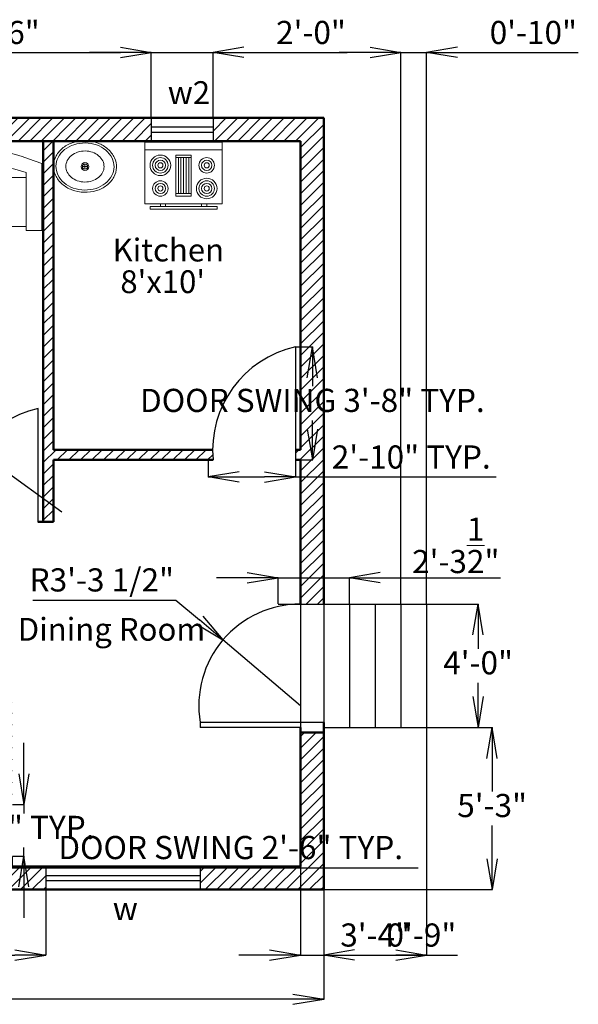
# Model space of a CAD drawing. Units: inches. Extents: x 1856 to 3350, y 1624 to 2224.
# Tile 3 of 7: x 2159 to 2376, y 1782 to 2165. Entities that reach past the tile are written whole.
import ezdxf

# ---------------------------------------------------------------- set-up
doc = ezdxf.new("R2010")
doc.units = ezdxf.units.IN
for name, color, linetype, lineweight in [('A-ANNO-DIMS', 2, 'Continuous', 18), ('A-ANNO-TEXT', 7, 'Continuous', 18), ('A-AREA-IDEN', 7, 'Continuous', 25), ('A-DOOR', 3, 'Continuous', 25), ('A-EQPM', 3, 'Continuous', 18), ('A-FLOR-FIXT', 3, 'Continuous', 18), ('A-FLOR-STRS', 7, 'Continuous', 25), ('A-FURN', 3, 'Continuous', 18), ('A-WALL', 7, 'Continuous', 50), ('A-WALL-PATT', 8, 'Continuous', 13), ('window', 4, 'Continuous', 25)]:
    doc.layers.add(name, color=color, linetype=linetype, lineweight=lineweight)
doc.styles.get("Standard").update_dxf_attribs({"font": 'arial.ttf'})
doc.dimstyles.new('ISO-25', dxfattribs={"dimtxt": 9, "dimasz": 12, "dimexe": 0.125, "dimexo": 0.125, "dimgap": 2, "dimtad": 1, "dimtih": 1, "dimtoh": 1, "dimdec": 1, "dimzin": 11, "dimlunit": 4, "dimtxsty": 'Standard', "dimblk": 'OPEN', "dimcen": -0.125, "dimadec": 0, "dimazin": 0, "dimtfac": 1, "dimtdec": 1, "dimtmove": 0, "dimatfit": 3, "dimfxl": 1, "dimarcsym": 0})

# ---------------------------------------------------------------- blocks, each defined once
blk = doc.blocks.new('_Open')
at = {"color": 0, "linetype": 'ByBlock', "lineweight": -2}
for p, q in [((-1, 0.167), (0, 0)), ((-1, -0.167), (0, 0)), ((0, 0), (-1, 0))]:
    blk.add_line(p, q, dxfattribs=at)
blk = doc.blocks.new('*D2')
at = {"layer": 'A-ANNO-DIMS', "color": 0, "lineweight": -2, "transparency": 16777216}
for p, q in [((2317.24, 1937.99), (2337.23, 1937.99)), ((2337.11, 1925.99), (2337.11, 1920.59)), ((2337.11, 1901.99), (2337.11, 1907.4)), ((2317.24, 1889.99), (2337.23, 1889.99))]:
    blk.add_line(p, q, dxfattribs=at)
at = {"layer": 'Defpoints', "color": 0, "transparency": 16777216}
for p in [(2317.11, 1937.99), (2317.11, 1889.99), (2337.11, 1889.99)]:
    blk.add_point(p, dxfattribs=at)
at = {"layer": 'A-ANNO-DIMS', "color": 0, "lineweight": -2, "transparency": 16777216, "xscale": 12, "yscale": 12, "zscale": 12}
for p, rotation in [((2337.11, 1937.99), 90), ((2337.11, 1889.99), 270)]:
    blk.add_blockref('_Open', p, dxfattribs=dict(at, rotation=rotation))
at = {"layer": 'A-ANNO-DIMS', "color": 0, "transparency": 16777216, "insert": (2337.11, 1913.99), "char_height": 9, "attachment_point": 5}
blk.add_mtext('4\'-0"', dxfattribs=at)
blk = doc.blocks.new('*D3')
at = {"layer": 'A-ANNO-DIMS', "color": 0, "lineweight": -2, "transparency": 16777216}
for p, q in [((2247.41, 1948.19), (2235.41, 1948.19)), ((2259.41, 1938.12), (2259.41, 1948.31)), ((2259.41, 1948.19), (2287.11, 1948.19)), ((2287.11, 1938.12), (2287.11, 1948.31)), ((2299.11, 1948.19), (2345.75, 1948.19))]:
    blk.add_line(p, q, dxfattribs=at)
at = {"layer": 'Defpoints', "color": 0, "transparency": 16777216}
for p in [(2287.11, 1948.19), (2259.41, 1937.99), (2287.11, 1937.99)]:
    blk.add_point(p, dxfattribs=at)
at = {"layer": 'A-ANNO-DIMS', "color": 0, "lineweight": -2, "transparency": 16777216, "xscale": 12, "yscale": 12, "zscale": 12}
blk.add_blockref('_Open', (2259.41, 1948.19), dxfattribs=at)
at = {"layer": 'A-ANNO-DIMS', "color": 0, "lineweight": -2, "transparency": 16777216, "xscale": 12, "yscale": 12, "zscale": 12, "rotation": 180}
blk.add_blockref('_Open', (2287.11, 1948.19), dxfattribs=at)
at = {"layer": 'A-ANNO-DIMS', "color": 0, "transparency": 16777216, "insert": (2328.43, 1960.81), "char_height": 9, "attachment_point": 5}
blk.add_mtext('2\'-3{\\H1x;\\S1/2;}"', dxfattribs=at)
blk = doc.blocks.new('*D7')
at = {"layer": 'A-ANNO-DIMS', "color": 0, "lineweight": -2, "transparency": 16777216}
for p, q in [((1923.11, 1826.87), (1923.11, 1784.25)), ((2277.11, 1826.87), (2277.11, 1784.25)), ((2265.11, 1784.37), (1935.11, 1784.37))]:
    blk.add_line(p, q, dxfattribs=at)
at = {"layer": 'Defpoints', "color": 0, "transparency": 16777216}
for p in [(1923.11, 1826.99), (2277.11, 1826.99), (1923.11, 1784.37)]:
    blk.add_point(p, dxfattribs=at)
at = {"layer": 'A-ANNO-DIMS', "color": 0, "lineweight": -2, "transparency": 16777216, "xscale": 12, "yscale": 12, "zscale": 12, "rotation": 180}
blk.add_blockref('_Open', (1923.11, 1784.37), dxfattribs=at)
at = {"layer": 'A-ANNO-DIMS', "color": 0, "lineweight": -2, "transparency": 16777216, "xscale": 12, "yscale": 12, "zscale": 12}
blk.add_blockref('_Open', (2277.11, 1784.37), dxfattribs=at)
at = {"layer": 'A-ANNO-DIMS', "color": 0, "transparency": 16777216, "insert": (2100.11, 1790.97), "char_height": 9, "attachment_point": 5}
blk.add_mtext("30'", dxfattribs=at)
blk = doc.blocks.new('Range-Oven - 30 in top')
for p, q in [((0, -3), (30, -3)), ((12, -6), (18, -6)), ((13, -20), (13, -6)), ((14, -6), (14, -20)), ((15, -20), (15, -6)), ((16, -6), (16, -20)), ((17, -20), (17, -6)), ((18, -20), (12, -20)), ((6, -24), (6, -25)), ((8, -25), (8, -24)), ((22, -25), (22, -24)), ((24, -24), (24, -25))]:
    blk.add_line(p, q)
for points in [[(0, -24), (0, 0), (30, 0), (30, -24)], [(12, -21), (12, -5), (18, -5), (18, -21)], [(2, -26), (2, -25), (28, -25), (28, -26)]]:
    blk.add_lwpolyline(points, close=True)
for centre, radius in [((6, -9), 4), ((6, -9), 3), ((6, -9), 2), ((24, -9), 3), ((24, -9), 2), ((6, -9), 1), ((24, -9), 1), ((6, -18), 3), ((24, -18), 4), ((24, -18), 3), ((6, -18), 2), ((6, -18), 1), ((24, -18), 2), ((24, -18), 1)]:
    blk.add_circle(centre, radius)
blk = doc.blocks.new('Sink - Oval top')
for p, q in [((-1, 0), (1, 0)), ((0, 1), (0, -1))]:
    blk.add_line(p, q)
for points in [[(-12.23, 0.39, 0.117634), (-11.46, -3.36, 0.104469), (-8.88, -6.8, 0.090016), (-5.08, -9.07, 0.08192), (-0.32, -10.02, 0.08192), (4.49, -9.38, 0.090016), (8.42, -7.36, 0.104469), (11.22, -4.09, 0.117634), (12.23, -0.39, 0.117634), (11.46, 3.36, 0.104469), (8.88, 6.8, 0.090016), (5.08, 9.07, 0.08192), (0.32, 10.02, 0.08192), (-4.49, 9.38, 0.090016), (-8.42, 7.36, 0.104469), (-11.22, 4.09, 0.117634)], [(-11.29, 0.16, 0.118622), (-10.52, -3.25, 0.104678), (-8.07, -6.36, 0.089562), (-4.54, -8.37, 0.081185), (-0.13, -9.15, 0.081185), (4.3, -8.49, 0.089562), (7.89, -6.58, 0.104678), (10.42, -3.55, 0.118622), (11.29, -0.16, 0.118622), (10.52, 3.25, 0.104678), (8.07, 6.36, 0.089562), (4.54, 8.37, 0.081185), (0.13, 9.15, 0.081185), (-4.3, 8.49, 0.089562), (-7.89, 6.58, 0.104678), (-10.42, 3.55, 0.118622)], [(-7.42, 0.08, 0.118283), (-6.91, -2.17, 0.104607), (-5.29, -4.21, 0.089718), (-2.97, -5.53, 0.081436), (-0.07, -6.04, 0.081436), (2.84, -5.59, 0.089718), (5.2, -4.33, 0.104607), (6.86, -2.32, 0.118283), (7.42, -0.08, 0.118283), (6.91, 2.17, 0.104607), (5.29, 4.21, 0.089718), (2.97, 5.53, 0.081436), (0.07, 6.04, 0.081436), (-2.84, 5.59, 0.089718), (-5.2, 4.33, 0.104607), (-6.86, 2.32, 0.118283)]]:
    blk.add_lwpolyline(points, format="xyb", close=True)
for radius in [1.5, 1]:
    blk.add_circle((0, 0), radius)
blk = doc.blocks.new('Sofa - Roundback 7 ft.')
for p, q in [((-12.00002, -32.4421), (-12.00003, -6.5971)), ((11.99997, -32.4421), (11.99998, -6.5971)), ((-36.000027, -34), (-36.000027, -11.4696)), ((35.99998, -34), (35.99998, -11.4696)), ((-35.999844, -13.3819), (35.9998, -13.3819)), ((-36.000027, -32.4421), (35.99998, -32.4421))]:
    blk.add_line(p, q)
for points in [[(-36.000027, -34), (-42.000027, -34), (-42.000027, -8)], [(41.99998, -8), (41.99998, -34), (35.99998, -34)]]:
    blk.add_lwpolyline(points)
for centre, radius, start, end in [((0, -114.25), 114.25, 68.43141, 111.5686), ((-0.00001, -127.1968), 121.1968, 72.72033, 107.2797)]:
    blk.add_arc(centre, radius, start, end)
blk = doc.blocks.new('WIN-60')
for p, q in [((0, 9), (60, 9)), ((0, 9), (0, 0)), ((60, 9), (60, 0)), ((0, 5.5), (60, 5.5)), ((0, 3.5), (60, 3.5)), ((0, 0), (60, 0))]:
    blk.add_line(p, q)
blk = doc.blocks.new('DOOR-SWING-44')
blk.add_line((32.16, 44), (32.16, 0))
blk.add_arc((41.37, 3.67), 41.37, 102.8606, 185.0846)
blk = doc.blocks.new('*D58')
at = {"layer": 'A-ANNO-DIMS', "color": 0, "lineweight": -2, "transparency": 16777216}
for p, q in [((2266.24, 2037.99), (2272.84, 2037.99)), ((2272.71, 2025.99), (2272.71, 2022.65)), ((2272.71, 2005.99), (2272.71, 2009.33)), ((2266.24, 1993.99), (2272.84, 1993.99))]:
    blk.add_line(p, q, dxfattribs=at)
at = {"layer": 'Defpoints', "color": 0, "transparency": 16777216}
for p in [(2266.11, 2037.99), (2272.71, 2037.99), (2266.11, 1993.99)]:
    blk.add_point(p, dxfattribs=at)
at = {"layer": 'A-ANNO-DIMS', "color": 0, "lineweight": -2, "transparency": 16777216, "xscale": 12, "yscale": 12, "zscale": 12}
for p, rotation in [((2272.71, 2037.99), 90), ((2272.71, 1993.99), 270)]:
    blk.add_blockref('_Open', p, dxfattribs=dict(at, rotation=rotation))
at = {"layer": 'A-ANNO-DIMS', "color": 0, "transparency": 16777216, "insert": (2272.71, 2015.99), "char_height": 9, "attachment_point": 5}
blk.add_mtext('DOOR SWING 3\'-8" TYP.', dxfattribs=at)
blk = doc.blocks.new('*D59')
at = {"layer": 'A-ANNO-DIMS', "color": 0, "lineweight": -2, "transparency": 16777216}
for p, q in [((2232.28, 1993.87), (2232.28, 1987.27)), ((2266.11, 1993.87), (2266.11, 1987.27)), ((2244.28, 1987.39), (2254.11, 1987.39)), ((2266.11, 1987.39), (2344.12, 1987.39))]:
    blk.add_line(p, q, dxfattribs=at)
at = {"layer": 'Defpoints', "color": 0, "transparency": 16777216}
for p in [(2232.28, 1993.99), (2266.11, 1993.99), (2266.11, 1987.39)]:
    blk.add_point(p, dxfattribs=at)
at = {"layer": 'A-ANNO-DIMS', "color": 0, "lineweight": -2, "transparency": 16777216, "xscale": 12, "yscale": 12, "zscale": 12, "rotation": 180}
blk.add_blockref('_Open', (2232.28, 1987.39), dxfattribs=at)
at = {"layer": 'A-ANNO-DIMS', "color": 0, "lineweight": -2, "transparency": 16777216, "xscale": 12, "yscale": 12, "zscale": 12}
blk.add_blockref('_Open', (2266.11, 1987.39), dxfattribs=at)
at = {"layer": 'A-ANNO-DIMS', "color": 0, "transparency": 16777216, "insert": (2311.12, 1993.99), "char_height": 9, "attachment_point": 5}
blk.add_mtext('2\'-10" TYP.', dxfattribs=at)
blk = doc.blocks.new('*D60')
at = {"layer": 'A-ANNO-DIMS', "color": 0, "lineweight": -2, "transparency": 16777216}
for p, q in [((2126.11, 1839.87), (2126.11, 1835.37)), ((2156.11, 1839.87), (2156.11, 1835.37)), ((2138.11, 1835.49), (2144.11, 1835.49)), ((2156.11, 1835.49), (2313.84, 1835.49))]:
    blk.add_line(p, q, dxfattribs=at)
at = {"layer": 'Defpoints', "color": 0, "transparency": 16777216}
for p in [(2126.11, 1839.99), (2156.11, 1839.99), (2156.11, 1835.49)]:
    blk.add_point(p, dxfattribs=at)
at = {"layer": 'A-ANNO-DIMS', "color": 0, "lineweight": -2, "transparency": 16777216, "xscale": 12, "yscale": 12, "zscale": 12, "rotation": 180}
blk.add_blockref('_Open', (2126.11, 1835.49), dxfattribs=at)
at = {"layer": 'A-ANNO-DIMS', "color": 0, "lineweight": -2, "transparency": 16777216, "xscale": 12, "yscale": 12, "zscale": 12}
blk.add_blockref('_Open', (2156.11, 1835.49), dxfattribs=at)
at = {"layer": 'A-ANNO-DIMS', "color": 0, "transparency": 16777216, "insert": (2240.97, 1842.15), "char_height": 9, "attachment_point": 5}
blk.add_mtext('DOOR SWING 2\'-6" TYP.', dxfattribs=at)
blk = doc.blocks.new('*D61')
at = {"layer": 'A-ANNO-DIMS', "color": 0, "lineweight": -2, "transparency": 16777216}
for p, q in [((2160.61, 1871.99), (2160.61, 1883.99)), ((2156.24, 1859.99), (2160.74, 1859.99)), ((2160.61, 1859.99), (2160.61, 1856.59)), ((2160.61, 1839.99), (2160.61, 1843.4)), ((2156.24, 1839.99), (2160.74, 1839.99)), ((2160.61, 1827.99), (2160.61, 1815.99))]:
    blk.add_line(p, q, dxfattribs=at)
at = {"layer": 'Defpoints', "color": 0, "transparency": 16777216}
for p in [(2156.11, 1859.99), (2160.61, 1859.99), (2156.11, 1839.99)]:
    blk.add_point(p, dxfattribs=at)
at = {"layer": 'A-ANNO-DIMS', "color": 0, "lineweight": -2, "transparency": 16777216, "xscale": 12, "yscale": 12, "zscale": 12}
for p, rotation in [((2160.61, 1859.99), 270), ((2160.61, 1839.99), 90)]:
    blk.add_blockref('_Open', p, dxfattribs=dict(at, rotation=rotation))
at = {"layer": 'A-ANNO-DIMS', "color": 0, "transparency": 16777216, "insert": (2160.61, 1849.99), "char_height": 9, "attachment_point": 5}
blk.add_mtext('1\'-8" TYP.', dxfattribs=at)
blk = doc.blocks.new('*D62')
at = {"layer": 'A-ANNO-DIMS', "color": 0, "lineweight": -2, "transparency": 16777216}
for p, q in [((2277.11, 1889.87), (2277.11, 1801.42)), ((2317.11, 1889.87), (2317.11, 1801.42)), ((2289.11, 1801.54), (2305.11, 1801.54))]:
    blk.add_line(p, q, dxfattribs=at)
at = {"layer": 'Defpoints', "color": 0, "transparency": 16777216}
for p in [(2277.11, 1889.99), (2317.11, 1889.99), (2317.11, 1801.54)]:
    blk.add_point(p, dxfattribs=at)
at = {"layer": 'A-ANNO-DIMS', "color": 0, "lineweight": -2, "transparency": 16777216, "xscale": 12, "yscale": 12, "zscale": 12, "rotation": 180}
blk.add_blockref('_Open', (2277.11, 1801.54), dxfattribs=at)
at = {"layer": 'A-ANNO-DIMS', "color": 0, "lineweight": -2, "transparency": 16777216, "xscale": 12, "yscale": 12, "zscale": 12}
blk.add_blockref('_Open', (2317.11, 1801.54), dxfattribs=at)
at = {"layer": 'A-ANNO-DIMS', "color": 0, "transparency": 16777216, "insert": (2297.11, 1808.14), "char_height": 9, "attachment_point": 5}
blk.add_mtext('3\'-4"', dxfattribs=at)
blk = doc.blocks.new('*D63')
at = {"layer": 'A-ANNO-DIMS', "color": 0, "lineweight": -2, "transparency": 16777216}
for p, q in [((2295.11, 2152.44), (2283.11, 2152.44)), ((2307.11, 1938.12), (2307.11, 2152.57)), ((2307.11, 2152.44), (2317.11, 2152.44)), ((2317.11, 1938.12), (2317.11, 2152.57)), ((2329.11, 2152.44), (2376.03, 2152.44))]:
    blk.add_line(p, q, dxfattribs=at)
at = {"layer": 'Defpoints', "color": 0, "transparency": 16777216}
for p in [(2317.11, 2152.44), (2307.11, 1937.99), (2317.11, 1937.99)]:
    blk.add_point(p, dxfattribs=at)
at = {"layer": 'A-ANNO-DIMS', "color": 0, "lineweight": -2, "transparency": 16777216, "xscale": 12, "yscale": 12, "zscale": 12}
blk.add_blockref('_Open', (2307.11, 2152.44), dxfattribs=at)
at = {"layer": 'A-ANNO-DIMS', "color": 0, "lineweight": -2, "transparency": 16777216, "xscale": 12, "yscale": 12, "zscale": 12, "rotation": 180}
blk.add_blockref('_Open', (2317.11, 2152.44), dxfattribs=at)
at = {"layer": 'A-ANNO-DIMS', "color": 0, "transparency": 16777216, "insert": (2358.57, 2159.04), "char_height": 9, "attachment_point": 5}
blk.add_mtext('0\'-10"', dxfattribs=at)
blk = doc.blocks.new('*D64')
at = {"layer": 'A-ANNO-DIMS', "color": 0, "lineweight": -2, "transparency": 16777216}
for p, q in [((2268.11, 1937.87), (2268.11, 1801.42)), ((2277.11, 1937.87), (2277.11, 1801.42)), ((2256.11, 1801.54), (2244.11, 1801.54)), ((2268.11, 1801.54), (2277.11, 1801.54)), ((2289.11, 1801.54), (2329.04, 1801.54))]:
    blk.add_line(p, q, dxfattribs=at)
at = {"layer": 'Defpoints', "color": 0, "transparency": 16777216}
for p in [(2268.11, 1937.99), (2277.11, 1937.99), (2277.11, 1801.54)]:
    blk.add_point(p, dxfattribs=at)
at = {"layer": 'A-ANNO-DIMS', "color": 0, "lineweight": -2, "transparency": 16777216, "xscale": 12, "yscale": 12, "zscale": 12}
blk.add_blockref('_Open', (2268.11, 1801.54), dxfattribs=at)
at = {"layer": 'A-ANNO-DIMS', "color": 0, "lineweight": -2, "transparency": 16777216, "xscale": 12, "yscale": 12, "zscale": 12, "rotation": 180}
blk.add_blockref('_Open', (2277.11, 1801.54), dxfattribs=at)
at = {"layer": 'A-ANNO-DIMS', "color": 0, "transparency": 16777216, "insert": (2315.08, 1808.14), "char_height": 9, "attachment_point": 5}
blk.add_mtext('0\'-9"', dxfattribs=at)
blk = doc.blocks.new('*D66')
at = {"layer": 'A-ANNO-DIMS', "color": 0, "lineweight": -2, "transparency": 16777216}
for p, q in [((2096.3, 2127.12), (2096.3, 2152.57)), ((2108.3, 2152.44), (2198.14, 2152.44)), ((2210.14, 2127.12), (2210.14, 2152.57))]:
    blk.add_line(p, q, dxfattribs=at)
at = {"layer": 'Defpoints', "color": 0, "transparency": 16777216}
for p in [(2210.14, 2152.44), (2096.3, 2126.99), (2210.14, 2126.99)]:
    blk.add_point(p, dxfattribs=at)
at = {"layer": 'A-ANNO-DIMS', "color": 0, "lineweight": -2, "transparency": 16777216, "xscale": 12, "yscale": 12, "zscale": 12, "rotation": 180}
blk.add_blockref('_Open', (2096.3, 2152.44), dxfattribs=at)
at = {"layer": 'A-ANNO-DIMS', "color": 0, "lineweight": -2, "transparency": 16777216, "xscale": 12, "yscale": 12, "zscale": 12}
blk.add_blockref('_Open', (2210.14, 2152.44), dxfattribs=at)
at = {"layer": 'A-ANNO-DIMS', "color": 0, "transparency": 16777216, "insert": (2153.22, 2159.04), "char_height": 9, "attachment_point": 5}
blk.add_mtext('9\'-6"', dxfattribs=at)
blk = doc.blocks.new('*D67')
at = {"layer": 'A-ANNO-DIMS', "color": 0, "lineweight": -2, "transparency": 16777216}
for p, q in [((2198.14, 2152.44), (2186.14, 2152.44)), ((2210.14, 2127.12), (2210.14, 2152.57)), ((2210.14, 2152.44), (2234.14, 2152.44)), ((2234.14, 2127.12), (2234.14, 2152.57)), ((2246.14, 2152.44), (2286.22, 2152.44))]:
    blk.add_line(p, q, dxfattribs=at)
at = {"layer": 'Defpoints', "color": 0, "transparency": 16777216}
for p in [(2234.14, 2152.44), (2210.14, 2126.99), (2234.14, 2126.99)]:
    blk.add_point(p, dxfattribs=at)
at = {"layer": 'A-ANNO-DIMS', "color": 0, "lineweight": -2, "transparency": 16777216, "xscale": 12, "yscale": 12, "zscale": 12}
blk.add_blockref('_Open', (2210.14, 2152.44), dxfattribs=at)
at = {"layer": 'A-ANNO-DIMS', "color": 0, "lineweight": -2, "transparency": 16777216, "xscale": 12, "yscale": 12, "zscale": 12, "rotation": 180}
blk.add_blockref('_Open', (2234.14, 2152.44), dxfattribs=at)
at = {"layer": 'A-ANNO-DIMS', "color": 0, "transparency": 16777216, "insert": (2272.18, 2159.04), "char_height": 9, "attachment_point": 5}
blk.add_mtext('2\'-0"', dxfattribs=at)
blk = doc.blocks.new('*D70')
at = {"layer": 'A-ANNO-DIMS', "color": 0, "lineweight": -2, "transparency": 16777216}
for p, q in [((2104.11, 1826.87), (2104.11, 1801.42)), ((2169.11, 1826.87), (2169.11, 1801.42)), ((2116.11, 1801.54), (2157.11, 1801.54))]:
    blk.add_line(p, q, dxfattribs=at)
at = {"layer": 'Defpoints', "color": 0, "transparency": 16777216}
for p in [(2104.11, 1826.99), (2169.11, 1826.99), (2169.11, 1801.54)]:
    blk.add_point(p, dxfattribs=at)
at = {"layer": 'A-ANNO-DIMS', "color": 0, "lineweight": -2, "transparency": 16777216, "xscale": 12, "yscale": 12, "zscale": 12, "rotation": 180}
blk.add_blockref('_Open', (2104.11, 1801.54), dxfattribs=at)
at = {"layer": 'A-ANNO-DIMS', "color": 0, "lineweight": -2, "transparency": 16777216, "xscale": 12, "yscale": 12, "zscale": 12}
blk.add_blockref('_Open', (2169.11, 1801.54), dxfattribs=at)
at = {"layer": 'A-ANNO-DIMS', "color": 0, "transparency": 16777216, "insert": (2136.61, 1808.12), "char_height": 9, "attachment_point": 5}
blk.add_mtext('5\'-5"', dxfattribs=at)
blk = doc.blocks.new('*D73')
at = {"layer": 'A-ANNO-DIMS', "color": 0, "lineweight": -2, "transparency": 16777216}
for p, q in [((2277.24, 1889.99), (2342.69, 1889.99)), ((2342.56, 1877.99), (2342.56, 1865.09)), ((2342.56, 1838.99), (2342.56, 1851.9)), ((2277.24, 1826.99), (2342.69, 1826.99))]:
    blk.add_line(p, q, dxfattribs=at)
at = {"layer": 'Defpoints', "color": 0, "transparency": 16777216}
for p in [(2277.11, 1889.99), (2342.56, 1889.99), (2277.11, 1826.99)]:
    blk.add_point(p, dxfattribs=at)
at = {"layer": 'A-ANNO-DIMS', "color": 0, "lineweight": -2, "transparency": 16777216, "xscale": 12, "yscale": 12, "zscale": 12}
for p, rotation in [((2342.56, 1889.99), 90), ((2342.56, 1826.99), 270)]:
    blk.add_blockref('_Open', p, dxfattribs=dict(at, rotation=rotation))
at = {"layer": 'A-ANNO-DIMS', "color": 0, "transparency": 16777216, "insert": (2342.56, 1858.49), "char_height": 9, "attachment_point": 5}
blk.add_mtext('5\'-3"', dxfattribs=at)
blk = doc.blocks.new('*D89')
at = {"layer": 'A-ANNO-DIMS', "color": 0, "lineweight": -2, "transparency": 16777216}
for p, q in [((2164.14, 1939.55), (2219.65, 1939.55)), ((2219.65, 1939.55), (2228.81, 1931.79)), ((2268.11, 1898.46), (2237.96, 1924.03))]:
    blk.add_line(p, q, dxfattribs=at)
at = {"layer": 'Defpoints', "color": 0, "transparency": 16777216}
for p in [(2237.96, 1924.03), (2268.11, 1898.46)]:
    blk.add_point(p, dxfattribs=at)
at = {"layer": 'A-ANNO-DIMS', "color": 0, "lineweight": -2, "transparency": 16777216, "xscale": 12, "yscale": 12, "zscale": 12, "rotation": 319.7083935961783}
blk.add_blockref('_Open', (2237.96, 1924.03), dxfattribs=at)
at = {"layer": 'A-ANNO-DIMS', "color": 0, "transparency": 16777216, "insert": (2190.9, 1946.2), "char_height": 9, "attachment_point": 5}
blk.add_mtext('R3\'-3 1/2"', dxfattribs=at)
blk = doc.blocks.new('*D91')
at = {"layer": 'A-ANNO-DIMS', "color": 0, "lineweight": -2, "transparency": 16777216}
for p, q in [((2046.79, 2012.59), (2121.79, 2012.59)), ((2121.79, 2012.59), (2132.16, 2005.05)), ((2175.32, 1973.66), (2141.86, 1997.99))]:
    blk.add_line(p, q, dxfattribs=at)
at = {"layer": 'Defpoints', "color": 0, "transparency": 16777216}
for p in [(2141.86, 1997.99), (2175.32, 1973.66)]:
    blk.add_point(p, dxfattribs=at)
at = {"layer": 'A-ANNO-DIMS', "color": 0, "lineweight": -2, "transparency": 16777216, "xscale": 12, "yscale": 12, "zscale": 12, "rotation": 323.9723172818348}
blk.add_blockref('_Open', (2141.86, 1997.99), dxfattribs=at)
at = {"layer": 'A-ANNO-DIMS', "color": 0, "transparency": 16777216, "insert": (2083.29, 2019.25), "char_height": 9, "attachment_point": 5}
blk.add_mtext('2X R3\'-5 1/2"', dxfattribs=at)

msp = doc.modelspace()

# ---------------------------------------------------------------- hatches: boundary and pattern name
at = {"layer": 'A-WALL-PATT'}
h = msp.add_hatch(dxfattribs=at)
h.set_pattern_fill('ANSI31', color=256)
h.paths.add_polyline_path([(2210.14, 2126.99), (2096.3, 2126.99), (2096.3, 2117.99), (2210.14, 2117.99)])
h.paths.add_polyline_path([(2048.3, 2126.99), (1923.11, 2126.99), (1923.11, 2077.99), (1932.11, 2077.99), (1932.11, 2117.99), (2006.11, 2117.99), (2008.11, 2117.99), (2008.11, 2113.99), (2012.11, 2113.99), (2012.11, 2117.99), (2048.29, 2117.99)])
h.paths.add_polyline_path([(2277.11, 2126.99), (2234.14, 2126.99), (2234.14, 2117.99), (2268.11, 2117.99), (2268.11, 1997.99), (2266.11, 1997.99), (2266.11, 1993.99), (2268.11, 1993.99), (2268.11, 1937.99), (2277.11, 1937.99)])
h.paths.add_polyline_path([(2277.11, 1887.99), (2268.11, 1887.99), (2268.11, 1835.99), (2229.11, 1835.99), (2229.11, 1826.99), (2277.11, 1826.99)])
h.paths.add_polyline_path([(2056.11, 1895.99), (2152.11, 1895.99), (2152.11, 1859.99), (2156.11, 1859.99), (2156.11, 1899.99), (2056.11, 1899.99), (2056.11, 1933.99), (2052.11, 1933.99), (2052.11, 1835.99), (2008.11, 1835.99), (2008.11, 1826.99), (2080.11, 1826.99), (2080.11, 1835.99), (2056.11, 1835.99)])
h.paths.add_polyline_path([(2169.11, 1835.99), (2156.11, 1835.99), (2156.11, 1837.99), (2152.11, 1837.99), (2152.11, 1835.99), (2104.11, 1835.99), (2104.11, 1826.99), (2169.11, 1826.99)])
h.paths.add_polyline_path([(1932.11, 1893.99), (1923.11, 1893.99), (1923.11, 1826.99), (1960.11, 1826.99), (1960.11, 1835.99), (1932.11, 1835.99)])
h.paths.add_polyline_path([(1932.11, 2013.99), (2008.11, 2013.99), (2008.11, 2017.99), (1932.11, 2017.99), (1932.11, 2053.99), (1923.11, 2053.99), (1923.11, 1941.99), (1932.11, 1941.99)])
h.paths.add_polyline_path([(2012.11, 2093.99, -0.030857), (2008.11, 2094.24), (2008.11, 1969.99), (2048.11, 1969.99), (2048.12, 1973.99), (2012.11, 1973.99)])
h.paths.add_polyline_path([(2172.11, 2117.99), (2168.11, 2117.99), (2168.11, 1969.99), (2172.11, 1969.99), (2172.11, 1993.99), (2234.11, 1993.99, -0.024205), (2233.95, 1997.99), (2172.11, 1997.99)])
h.paths.add_polyline_path([(2133.95, 1973.99), (2048.12, 1973.99), (2048.11, 1969.99), (2052.11, 1969.99), (2052.11, 1967.99), (2056.11, 1967.99), (2056.11, 1969.99), (2134.11, 1969.99, -0.024205)])

# ---------------------------------------------------------------- linework, layer by layer
at = {"layer": 'A-DOOR'}
for p, q in [((2266.11, 2037.99), (2266.11, 1997.99)), ((2229.11, 1891.99), (2229.11, 1889.99)), ((2277.11, 1891.99), (2229.11, 1891.99)), ((2268.11, 1889.99), (2229.11, 1889.99))]:
    msp.add_line(p, q, dxfattribs=at)
msp.add_arc((2268.11, 1898.46), 39.53, 90, 189.4157, dxfattribs=at)
at = {"layer": 'A-FLOR-STRS'}
for p, q in [((2259.41, 1937.99), (2317.11, 1937.99)), ((2277.11, 1937.99), (2277.11, 1889.99)), ((2287.11, 1937.99), (2287.11, 1889.99)), ((2297.11, 1937.99), (2297.11, 1889.99)), ((2307.11, 1937.99), (2307.11, 1889.99)), ((2317.11, 1937.99), (2317.11, 1889.99)), ((2277.11, 1889.99), (2317.11, 1889.99))]:
    msp.add_line(p, q, dxfattribs=at)
at = {"layer": 'A-WALL'}
for p, q in [((1923.11, 2126.99), (2277.11, 2126.99)), ((2277.11, 2126.99), (2277.11, 1937.99)), ((2012.11, 2117.99), (2268.11, 2117.99)), ((2168.11, 2117.99), (2168.11, 1969.99)), ((2172.11, 2117.99), (2172.11, 1997.99)), ((2268.11, 2117.99), (2268.11, 1997.99)), ((2172.11, 1997.99), (2233.95, 1997.99)), ((2266.11, 1997.99), (2268.11, 1997.99)), ((2172.11, 1993.99), (2234.11, 1993.99)), ((2172.11, 1993.99), (2172.11, 1969.99)), ((2266.11, 1993.99), (2268.11, 1993.99)), ((2268.11, 1993.99), (2268.11, 1937.99)), ((2166.11, 1969.99), (2172.11, 1969.99)), ((2277.11, 1891.99), (2277.11, 1826.99)), ((2268.11, 1889.99), (2268.11, 1835.99)), ((2277.11, 1887.99), (2268.11, 1887.99)), ((2268.11, 1835.99), (2156.11, 1835.99)), ((2277.11, 1826.99), (1923.11, 1826.99))]:
    msp.add_line(p, q, dxfattribs=at)
at = {"layer": 'window'}
for p, q in [((2210.14, 2126.99), (2234.14, 2126.99)), ((2210.14, 2126.99), (2210.14, 2117.99)), ((2234.14, 2126.99), (2234.14, 2117.99)), ((2234.14, 2126.99), (2234.14, 2117.99)), ((2210.14, 2123.49), (2234.14, 2123.49)), ((2210.14, 2121.49), (2234.14, 2121.49)), ((2210.14, 2117.99), (2234.14, 2117.99)), ((2229.11, 1835.99), (2229.11, 1826.99))]:
    msp.add_line(p, q, dxfattribs=at)

# ---------------------------------------------------------------- block references
at = {"layer": 'A-DOOR'}
for p in [(2233.95, 1993.99), (2133.95, 1969.99)]:
    msp.add_blockref('DOOR-SWING-44', p, dxfattribs=at)
at = {"layer": 'A-EQPM'}
msp.add_blockref('Range-Oven - 30 in top', (2207.66, 2117.55), dxfattribs=at)
at = {"layer": 'A-FLOR-FIXT'}
msp.add_blockref('Sink - Oval top', (2184.36, 2108.09), dxfattribs=at)
at = {"layer": 'A-FURN'}
msp.add_blockref('Sofa - Roundback 7 ft.', (2125.57, 2117.22), dxfattribs=at)
at = {"layer": 'window'}
msp.add_blockref('WIN-60', (2169.11, 1826.99), dxfattribs=at)

# ---------------------------------------------------------------- texts
at = {"layer": 'A-ANNO-TEXT'}
for s, height, p in [('w2', 8.871, (2216.56, 2132.38)), ('w', 8.87, (2195.18, 1815.16))]:
    msp.add_text(s, height=height, dxfattribs=at).set_placement(p)
at = {"layer": 'A-AREA-IDEN'}
for s, height, p in [('Kitchen', 8.871, (2195.1, 2071.18)), ("  8'x10'", 8.871, (2192.68, 2058.87)), ('Dining Room', 8.8713, (2158.23, 1923.72))]:
    msp.add_text(s, height=height, dxfattribs=at).set_placement(p)

# ---------------------------------------------------------------- dimensions: what is measured, and where the dimension line sits
at = {"layer": 'A-ANNO-DIMS'}
for base, p1, p2, override, picture, middle in [((2210.14, 2152.44), (2096.3, 2126.99), (2210.14, 2126.99), {"dimdec": 1, "dimlfac": 1, "dimrnd": 0, "dimzin": 1, "dimdsep": 46, "dimlunit": 4, "dimfrac": 2}, '*D66', (2153.22, 2159.04)), ((2234.14, 2152.44), (2210.14, 2126.99), (2234.14, 2126.99), {"dimdec": 1, "dimlfac": 1, "dimrnd": 0, "dimzin": 1, "dimdsep": 46, "dimlunit": 4, "dimfrac": 2}, '*D67', (2272.18, 2159.04)), ((2317.11, 2152.44), (2307.11, 1937.99), (2317.11, 1937.99), {"dimdec": 1, "dimlfac": 1, "dimrnd": 0, "dimzin": 1, "dimdsep": 46, "dimlunit": 4, "dimfrac": 2}, '*D63', (2358.57, 2159.04)), ((2287.11, 1948.19), (2259.41, 1937.99), (2287.11, 1937.99), {"dimclrd": 0, "dimclre": 0, "dimclrt": 0}, '*D3', (2328.43, 1960.81)), ((2277.11, 1801.54), (2268.11, 1937.99), (2277.11, 1937.99), {"dimdec": 1, "dimlfac": 1, "dimrnd": 0, "dimzin": 1, "dimdsep": 46, "dimlunit": 4, "dimfrac": 2}, '*D64', (2315.08, 1808.14)), ((2317.11, 1801.54), (2277.11, 1889.99), (2317.11, 1889.99), {"dimdec": 1, "dimlfac": 1, "dimrnd": 0, "dimzin": 1, "dimdsep": 46, "dimlunit": 4, "dimfrac": 2}, '*D62', (2297.11, 1808.14)), ((2169.11, 1801.54), (2104.11, 1826.99), (2169.11, 1826.99), {"dimdec": 1, "dimlfac": 1, "dimrnd": 0, "dimzin": 1, "dimdsep": 46, "dimlunit": 4, "dimfrac": 2}, '*D70', (2136.61, 1808.12))]:
    dim = msp.add_linear_dim(base=base, p1=p1, p2=p2, dimstyle='ISO-25', override=override, dxfattribs=at)
    dim.commit()
    dim.dimension.update_dxf_attribs({"geometry": picture, "text_midpoint": middle})
for base, p1, p2, text, picture, middle in [((2272.71, 2037.99), (2266.11, 1993.99), (2266.11, 2037.99), 'DOOR SWING <> TYP.', '*D58', (2272.71, 2015.99)), ((2160.61, 1859.99), (2156.11, 1839.99), (2156.11, 1859.99), '<> TYP.', '*D61', (2160.61, 1849.99))]:
    dim = msp.add_linear_dim(base=base, p1=p1, p2=p2, angle=90, text=text, dimstyle='ISO-25', override={"dimdec": 1, "dimlfac": 1, "dimrnd": 0, "dimzin": 1, "dimdsep": 46, "dimlunit": 4, "dimfrac": 2}, dxfattribs=at)
    dim.commit()
    dim.dimension.update_dxf_attribs({"geometry": picture, "text_midpoint": middle})
dim = msp.add_radius_dim(center=(2175.32, 1973.66), mpoint=(2141.86, 1997.99), text='2X <>', dimstyle='ISO-25', override={"dimdec": 1, "dimlfac": 1, "dimrnd": 0, "dimzin": 1, "dimdsep": 46, "dimlunit": 4, "dimfrac": 2}, dxfattribs=at)
dim.commit()
dim.dimension.update_dxf_attribs({"geometry": '*D91', "text_midpoint": (2083.29, 2012.59), "dimtype": 164})
for base, p1, p2, text, override, picture, middle in [((2266.11, 1987.39), (2232.28, 1993.99), (2266.11, 1993.99), '<> TYP.', {"dimdec": 1, "dimlfac": 1, "dimrnd": 0, "dimzin": 1, "dimdsep": 46, "dimlunit": 4, "dimfrac": 2}, '*D59', (2311.12, 1993.99)), ((2156.11, 1835.49), (2126.11, 1839.99), (2156.11, 1839.99), 'DOOR SWING <> TYP.', {"dimdec": 1, "dimlfac": 1, "dimrnd": 0, "dimzin": 1, "dimdsep": 46, "dimlunit": 4, "dimfrac": 2}, '*D60', (2240.97, 1842.15)), ((1923.11, 1784.37), (2277.11, 1826.99), (1923.11, 1826.99), "30'", {"dimclrd": 0, "dimclre": 0, "dimclrt": 0}, '*D7', (2100.11, 1790.97))]:
    dim = msp.add_linear_dim(base=base, p1=p1, p2=p2, text=text, dimstyle='ISO-25', override=override, dxfattribs=at)
    dim.commit()
    dim.dimension.update_dxf_attribs({"geometry": picture, "text_midpoint": middle})
dim = msp.add_radius_dim(center=(2268.11, 1898.46), mpoint=(2237.96, 1924.03), dimstyle='ISO-25', override={"dimdec": 1, "dimlfac": 1, "dimrnd": 0, "dimzin": 1, "dimdsep": 46, "dimlunit": 4, "dimfrac": 2}, dxfattribs=at)
dim.commit()
dim.dimension.update_dxf_attribs({"geometry": '*D89', "text_midpoint": (2190.9, 1946.2)})
for base, p1, p2, override, picture, middle in [((2337.11, 1889.99), (2317.11, 1937.99), (2317.11, 1889.99), {"dimclrd": 0, "dimclre": 0, "dimclrt": 0}, '*D2', (2337.11, 1913.99)), ((2342.56, 1889.99), (2277.11, 1826.99), (2277.11, 1889.99), {"dimdec": 1, "dimlfac": 1, "dimrnd": 0, "dimzin": 1, "dimdsep": 46, "dimlunit": 4, "dimfrac": 2}, '*D73', (2342.56, 1858.49))]:
    dim = msp.add_linear_dim(base=base, p1=p1, p2=p2, angle=90, dimstyle='ISO-25', override=override, dxfattribs=at)
    dim.commit()
    dim.dimension.update_dxf_attribs({"geometry": picture, "text_midpoint": middle})

doc.saveas('drawing.dxf')
